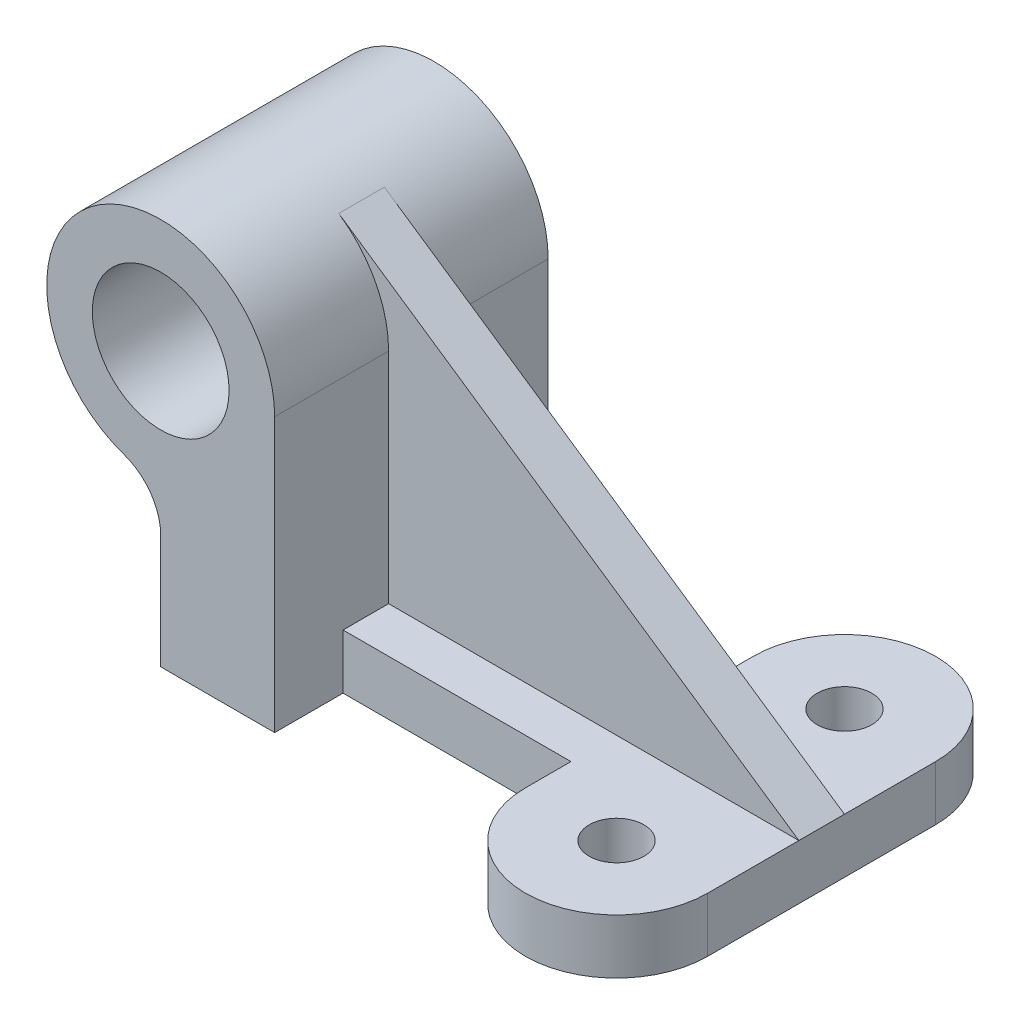
ISO-10303-21;
HEADER;
FILE_DESCRIPTION(('STEP AP214'),'2;1');
FILE_NAME('part.step','',(''),(''),'','','');
FILE_SCHEMA(('AUTOMOTIVE_DESIGN { 1 0 10303 214 1 1 1 1 }'));
ENDSEC;
DATA;
#1=APPLICATION_CONTEXT('core data for automotive mechanical design processes');
#2=APPLICATION_PROTOCOL_DEFINITION('international standard','automotive_design',2000,#1);
#3=PRODUCT_CONTEXT('',#1,'mechanical');
#4=PRODUCT('Part','Part','',(#3));
#5=PRODUCT_RELATED_PRODUCT_CATEGORY('part','',(#4));
#6=PRODUCT_DEFINITION_FORMATION('','',#4);
#7=PRODUCT_DEFINITION_CONTEXT('part definition',#1,'design');
#8=PRODUCT_DEFINITION('design','',#6,#7);
#9=PRODUCT_DEFINITION_SHAPE('','',#8);
#10=(LENGTH_UNIT() NAMED_UNIT(*) SI_UNIT(.MILLI.,.METRE.));
#11=(NAMED_UNIT(*) PLANE_ANGLE_UNIT() SI_UNIT($,.RADIAN.));
#12=(NAMED_UNIT(*) SI_UNIT($,.STERADIAN.) SOLID_ANGLE_UNIT());
#13=UNCERTAINTY_MEASURE_WITH_UNIT(LENGTH_MEASURE(1.E-05),#10,'distance_accuracy_value','');
#14=(GEOMETRIC_REPRESENTATION_CONTEXT(3) GLOBAL_UNCERTAINTY_ASSIGNED_CONTEXT((#13)) GLOBAL_UNIT_ASSIGNED_CONTEXT((#10,
#11,#12)) REPRESENTATION_CONTEXT('',''));
#15=CARTESIAN_POINT('',(0.,0.,0.));
#16=DIRECTION('',(0.,0.,1.));
#17=DIRECTION('',(1.,0.,0.));
#18=AXIS2_PLACEMENT_3D('',#15,#16,#17);
#19=CARTESIAN_POINT('',(0.,6.,25.));
#20=DIRECTION('',(0.,1.,0.));
#21=DIRECTION('',(0.,0.,1.));
#22=AXIS2_PLACEMENT_3D('',#19,#20,#21);
#23=PLANE('',#22);
#24=CARTESIAN_POINT('',(0.,6.,-25.));
#25=DIRECTION('',(0.,1.,0.));
#26=DIRECTION('',(0.,0.,1.));
#27=AXIS2_PLACEMENT_3D('',#24,#25,#26);
#28=CIRCLE('',#27,6.);
#29=CARTESIAN_POINT('',(0.,6.,-19.));
#30=VERTEX_POINT('',#29);
#31=EDGE_CURVE('E241',#30,#30,#28,.T.);
#32=ORIENTED_EDGE('',*,*,#31,.F.);
#33=EDGE_LOOP('',(#32));
#34=FACE_BOUND('',#33,.T.);
#35=DIRECTION('',(0.,0.,1.));
#36=VECTOR('',#35,1.);
#37=CARTESIAN_POINT('',(-70.,6.,-15.));
#38=LINE('',#37,#36);
#39=CARTESIAN_POINT('',(-70.,6.,-15.));
#40=VERTEX_POINT('',#39);
#41=CARTESIAN_POINT('',(-70.,6.,-5.));
#42=VERTEX_POINT('',#41);
#43=EDGE_CURVE('E259',#40,#42,#38,.T.);
#44=ORIENTED_EDGE('',*,*,#43,.T.);
#45=DIRECTION('',(1.,0.,0.));
#46=VECTOR('',#45,1.);
#47=CARTESIAN_POINT('',(0.,6.,-5.));
#48=LINE('',#47,#46);
#49=CARTESIAN_POINT('',(20.,6.,-5.));
#50=VERTEX_POINT('',#49);
#51=EDGE_CURVE('E59',#42,#50,#48,.T.);
#52=ORIENTED_EDGE('',*,*,#51,.T.);
#53=DIRECTION('',(0.,0.,-1.));
#54=VECTOR('',#53,1.);
#55=CARTESIAN_POINT('',(20.,6.,-25.));
#56=LINE('',#55,#54);
#57=CARTESIAN_POINT('',(20.,6.,-25.));
#58=VERTEX_POINT('',#57);
#59=EDGE_CURVE('E270',#50,#58,#56,.T.);
#60=ORIENTED_EDGE('',*,*,#59,.T.);
#61=CARTESIAN_POINT('',(0.,6.,-25.));
#62=DIRECTION('',(0.,1.,0.));
#63=DIRECTION('',(0.,0.,1.));
#64=AXIS2_PLACEMENT_3D('',#61,#62,#63);
#65=CIRCLE('',#64,20.);
#66=CARTESIAN_POINT('',(-20.,6.,-25.));
#67=VERTEX_POINT('',#66);
#68=EDGE_CURVE('E269',#58,#67,#65,.T.);
#69=ORIENTED_EDGE('',*,*,#68,.T.);
#70=DIRECTION('',(0.,0.,1.));
#71=VECTOR('',#70,1.);
#72=CARTESIAN_POINT('',(-20.,6.,-25.));
#73=LINE('',#72,#71);
#74=CARTESIAN_POINT('',(-20.,6.,-15.));
#75=VERTEX_POINT('',#74);
#76=EDGE_CURVE('E253',#67,#75,#73,.T.);
#77=ORIENTED_EDGE('',*,*,#76,.T.);
#78=DIRECTION('',(-1.,0.,0.));
#79=VECTOR('',#78,1.);
#80=CARTESIAN_POINT('',(-70.,6.,-15.));
#81=LINE('',#80,#79);
#82=EDGE_CURVE('E255',#75,#40,#81,.T.);
#83=ORIENTED_EDGE('',*,*,#82,.T.);
#84=EDGE_LOOP('',(#44,#52,#60,#69,#77,#83));
#85=FACE_BOUND('',#84,.T.);
#86=ADVANCED_FACE('F43',(#34,#85),#23,.T.);
#87=CARTESIAN_POINT('',(-70.,-6.,30.));
#88=DIRECTION('',(-1.,0.,0.));
#89=DIRECTION('',(0.,0.,1.));
#90=AXIS2_PLACEMENT_3D('',#87,#88,#89);
#91=PLANE('',#90);
#92=DIRECTION('',(0.,1.,0.));
#93=VECTOR('',#92,1.);
#94=CARTESIAN_POINT('',(-70.,-6.,-5.));
#95=LINE('',#94,#93);
#96=CARTESIAN_POINT('',(-70.,54.,-5.));
#97=VERTEX_POINT('',#96);
#98=EDGE_CURVE('E177',#42,#97,#95,.T.);
#99=ORIENTED_EDGE('',*,*,#98,.F.);
#100=ORIENTED_EDGE('',*,*,#43,.F.);
#101=DIRECTION('',(0.,-1.,0.));
#102=VECTOR('',#101,1.);
#103=CARTESIAN_POINT('',(-70.,6.,-15.));
#104=LINE('',#103,#102);
#105=CARTESIAN_POINT('',(-70.,-6.,-15.));
#106=VERTEX_POINT('',#105);
#107=EDGE_CURVE('E303',#40,#106,#104,.T.);
#108=ORIENTED_EDGE('',*,*,#107,.T.);
#109=DIRECTION('',(0.,0.,-1.));
#110=VECTOR('',#109,1.);
#111=CARTESIAN_POINT('',(-70.,-6.,30.));
#112=LINE('',#111,#110);
#113=CARTESIAN_POINT('',(-70.,-6.,-30.));
#114=VERTEX_POINT('',#113);
#115=EDGE_CURVE('E213',#106,#114,#112,.T.);
#116=ORIENTED_EDGE('',*,*,#115,.T.);
#117=DIRECTION('',(0.,1.,0.));
#118=VECTOR('',#117,1.);
#119=CARTESIAN_POINT('',(-70.,-6.,-30.));
#120=LINE('',#119,#118);
#121=CARTESIAN_POINT('',(-70.,54.,-30.));
#122=VERTEX_POINT('',#121);
#123=EDGE_CURVE('E196',#114,#122,#120,.T.);
#124=ORIENTED_EDGE('',*,*,#123,.T.);
#125=DIRECTION('',(0.,0.,-1.));
#126=VECTOR('',#125,1.);
#127=CARTESIAN_POINT('',(-70.,54.,30.));
#128=LINE('',#127,#126);
#129=EDGE_CURVE('E234',#97,#122,#128,.T.);
#130=ORIENTED_EDGE('',*,*,#129,.F.);
#131=EDGE_LOOP('',(#99,#100,#108,#116,#124,#130));
#132=FACE_BOUND('',#131,.T.);
#133=ADVANCED_FACE('F323',(#132),#91,.F.);
#134=DIRECTION('',(1.,0.,0.));
#135=VECTOR('',#134,1.);
#136=CARTESIAN_POINT('',(0.,6.,5.));
#137=LINE('',#136,#135);
#138=CARTESIAN_POINT('',(-70.,6.,5.));
#139=VERTEX_POINT('',#138);
#140=CARTESIAN_POINT('',(20.,6.,5.));
#141=VERTEX_POINT('',#140);
#142=EDGE_CURVE('E186',#139,#141,#137,.T.);
#143=ORIENTED_EDGE('',*,*,#142,.F.);
#144=CARTESIAN_POINT('',(-70.,6.,15.));
#145=VERTEX_POINT('',#144);
#146=EDGE_CURVE('E256',#139,#145,#38,.T.);
#147=ORIENTED_EDGE('',*,*,#146,.T.);
#148=DIRECTION('',(1.,0.,0.));
#149=VECTOR('',#148,1.);
#150=CARTESIAN_POINT('',(-70.,6.,15.));
#151=LINE('',#150,#149);
#152=CARTESIAN_POINT('',(-20.,6.,15.));
#153=VERTEX_POINT('',#152);
#154=EDGE_CURVE('E261',#145,#153,#151,.T.);
#155=ORIENTED_EDGE('',*,*,#154,.T.);
#156=DIRECTION('',(0.,0.,1.));
#157=VECTOR('',#156,1.);
#158=CARTESIAN_POINT('',(-20.,6.,15.));
#159=LINE('',#158,#157);
#160=CARTESIAN_POINT('',(-20.,6.,25.));
#161=VERTEX_POINT('',#160);
#162=EDGE_CURVE('E263',#153,#161,#159,.T.);
#163=ORIENTED_EDGE('',*,*,#162,.T.);
#164=CARTESIAN_POINT('',(0.,6.,25.));
#165=DIRECTION('',(0.,1.,0.));
#166=DIRECTION('',(0.,0.,1.));
#167=AXIS2_PLACEMENT_3D('',#164,#165,#166);
#168=CIRCLE('',#167,20.);
#169=CARTESIAN_POINT('',(20.,6.,25.));
#170=VERTEX_POINT('',#169);
#171=EDGE_CURVE('E264',#161,#170,#168,.T.);
#172=ORIENTED_EDGE('',*,*,#171,.T.);
#173=EDGE_CURVE('E268',#170,#141,#56,.T.);
#174=ORIENTED_EDGE('',*,*,#173,.T.);
#175=EDGE_LOOP('',(#143,#147,#155,#163,#172,#174));
#176=FACE_BOUND('',#175,.T.);
#177=CARTESIAN_POINT('',(0.,6.,25.));
#178=DIRECTION('',(0.,1.,0.));
#179=DIRECTION('',(0.,0.,1.));
#180=AXIS2_PLACEMENT_3D('',#177,#178,#179);
#181=CIRCLE('',#180,6.);
#182=CARTESIAN_POINT('',(0.,6.,31.));
#183=VERTEX_POINT('',#182);
#184=EDGE_CURVE('E239',#183,#183,#181,.T.);
#185=ORIENTED_EDGE('',*,*,#184,.F.);
#186=EDGE_LOOP('',(#185));
#187=FACE_BOUND('',#186,.T.);
#188=ADVANCED_FACE('F385',(#176,#187),#23,.T.);
#189=CARTESIAN_POINT('',(0.,-6.,25.));
#190=DIRECTION('',(0.,1.,0.));
#191=DIRECTION('',(0.,0.,1.));
#192=AXIS2_PLACEMENT_3D('',#189,#190,#191);
#193=PLANE('',#192);
#194=DIRECTION('',(0.,0.,-1.));
#195=VECTOR('',#194,1.);
#196=CARTESIAN_POINT('',(-95.,-6.,30.));
#197=LINE('',#196,#195);
#198=CARTESIAN_POINT('',(-95.,-6.,30.));
#199=VERTEX_POINT('',#198);
#200=CARTESIAN_POINT('',(-95.,-6.,-30.));
#201=VERTEX_POINT('',#200);
#202=EDGE_CURVE('E230',#199,#201,#197,.T.);
#203=ORIENTED_EDGE('',*,*,#202,.T.);
#204=DIRECTION('',(1.,0.,0.));
#205=VECTOR('',#204,1.);
#206=CARTESIAN_POINT('',(-70.,-6.,-30.));
#207=LINE('',#206,#205);
#208=EDGE_CURVE('E202',#201,#114,#207,.T.);
#209=ORIENTED_EDGE('',*,*,#208,.T.);
#210=ORIENTED_EDGE('',*,*,#115,.F.);
#211=DIRECTION('',(-1.,0.,0.));
#212=VECTOR('',#211,1.);
#213=CARTESIAN_POINT('',(-70.,-6.,-15.));
#214=LINE('',#213,#212);
#215=CARTESIAN_POINT('',(-20.,-6.,-15.));
#216=VERTEX_POINT('',#215);
#217=EDGE_CURVE('E274',#216,#106,#214,.T.);
#218=ORIENTED_EDGE('',*,*,#217,.F.);
#219=DIRECTION('',(0.,0.,1.));
#220=VECTOR('',#219,1.);
#221=CARTESIAN_POINT('',(-20.,-6.,-25.));
#222=LINE('',#221,#220);
#223=CARTESIAN_POINT('',(-20.,-6.,-25.));
#224=VERTEX_POINT('',#223);
#225=EDGE_CURVE('E247',#224,#216,#222,.T.);
#226=ORIENTED_EDGE('',*,*,#225,.F.);
#227=CARTESIAN_POINT('',(0.,-6.,-25.));
#228=DIRECTION('',(0.,1.,0.));
#229=DIRECTION('',(0.,0.,1.));
#230=AXIS2_PLACEMENT_3D('',#227,#228,#229);
#231=CIRCLE('',#230,20.);
#232=CARTESIAN_POINT('',(20.,-6.,-25.));
#233=VERTEX_POINT('',#232);
#234=EDGE_CURVE('E254',#233,#224,#231,.T.);
#235=ORIENTED_EDGE('',*,*,#234,.F.);
#236=DIRECTION('',(0.,0.,-1.));
#237=VECTOR('',#236,1.);
#238=CARTESIAN_POINT('',(20.,-6.,-25.));
#239=LINE('',#238,#237);
#240=CARTESIAN_POINT('',(20.,-6.,25.));
#241=VERTEX_POINT('',#240);
#242=EDGE_CURVE('E285',#241,#233,#239,.T.);
#243=ORIENTED_EDGE('',*,*,#242,.F.);
#244=CARTESIAN_POINT('',(0.,-6.,25.));
#245=DIRECTION('',(0.,1.,0.));
#246=DIRECTION('',(0.,0.,1.));
#247=AXIS2_PLACEMENT_3D('',#244,#245,#246);
#248=CIRCLE('',#247,20.);
#249=CARTESIAN_POINT('',(-20.,-6.,25.));
#250=VERTEX_POINT('',#249);
#251=EDGE_CURVE('E284',#250,#241,#248,.T.);
#252=ORIENTED_EDGE('',*,*,#251,.F.);
#253=DIRECTION('',(0.,0.,1.));
#254=VECTOR('',#253,1.);
#255=CARTESIAN_POINT('',(-20.,-6.,15.));
#256=LINE('',#255,#254);
#257=CARTESIAN_POINT('',(-20.,-6.,15.));
#258=VERTEX_POINT('',#257);
#259=EDGE_CURVE('E278',#258,#250,#256,.T.);
#260=ORIENTED_EDGE('',*,*,#259,.F.);
#261=DIRECTION('',(1.,0.,0.));
#262=VECTOR('',#261,1.);
#263=CARTESIAN_POINT('',(-70.,-6.,15.));
#264=LINE('',#263,#262);
#265=CARTESIAN_POINT('',(-70.,-6.,15.));
#266=VERTEX_POINT('',#265);
#267=EDGE_CURVE('E279',#266,#258,#264,.T.);
#268=ORIENTED_EDGE('',*,*,#267,.F.);
#269=CARTESIAN_POINT('',(-70.,-6.,30.));
#270=VERTEX_POINT('',#269);
#271=EDGE_CURVE('E229',#270,#266,#112,.T.);
#272=ORIENTED_EDGE('',*,*,#271,.F.);
#273=DIRECTION('',(1.,0.,0.));
#274=VECTOR('',#273,1.);
#275=CARTESIAN_POINT('',(-70.,-6.,30.));
#276=LINE('',#275,#274);
#277=EDGE_CURVE('E211',#199,#270,#276,.T.);
#278=ORIENTED_EDGE('',*,*,#277,.F.);
#279=EDGE_LOOP('',(#203,#209,#210,#218,#226,#235,#243,#252,#260,#268,#272,#278));
#280=FACE_BOUND('',#279,.T.);
#281=CARTESIAN_POINT('',(0.,-6.,25.));
#282=DIRECTION('',(0.,1.,0.));
#283=DIRECTION('',(0.,0.,1.));
#284=AXIS2_PLACEMENT_3D('',#281,#282,#283);
#285=CIRCLE('',#284,6.);
#286=CARTESIAN_POINT('',(0.,-6.,31.));
#287=VERTEX_POINT('',#286);
#288=EDGE_CURVE('E236',#287,#287,#285,.T.);
#289=ORIENTED_EDGE('',*,*,#288,.T.);
#290=EDGE_LOOP('',(#289));
#291=FACE_BOUND('',#290,.T.);
#292=CARTESIAN_POINT('',(0.,-6.,-25.));
#293=DIRECTION('',(0.,1.,0.));
#294=DIRECTION('',(0.,0.,1.));
#295=AXIS2_PLACEMENT_3D('',#292,#293,#294);
#296=CIRCLE('',#295,6.);
#297=CARTESIAN_POINT('',(0.,-6.,-19.));
#298=VERTEX_POINT('',#297);
#299=EDGE_CURVE('E244',#298,#298,#296,.T.);
#300=ORIENTED_EDGE('',*,*,#299,.T.);
#301=EDGE_LOOP('',(#300));
#302=FACE_BOUND('',#301,.T.);
#303=ADVANCED_FACE('F316',(#280,#291,#302),#193,.F.);
#304=CARTESIAN_POINT('',(-20.,6.,-25.));
#305=DIRECTION('',(1.,0.,0.));
#306=DIRECTION('',(0.,0.,-1.));
#307=AXIS2_PLACEMENT_3D('',#304,#305,#306);
#308=PLANE('',#307);
#309=ORIENTED_EDGE('',*,*,#225,.T.);
#310=DIRECTION('',(0.,-1.,0.));
#311=VECTOR('',#310,1.);
#312=CARTESIAN_POINT('',(-20.,6.,-15.));
#313=LINE('',#312,#311);
#314=EDGE_CURVE('E51',#75,#216,#313,.T.);
#315=ORIENTED_EDGE('',*,*,#314,.F.);
#316=ORIENTED_EDGE('',*,*,#76,.F.);
#317=DIRECTION('',(0.,-1.,0.));
#318=VECTOR('',#317,1.);
#319=CARTESIAN_POINT('',(-20.,6.,-25.));
#320=LINE('',#319,#318);
#321=EDGE_CURVE('E275',#67,#224,#320,.T.);
#322=ORIENTED_EDGE('',*,*,#321,.T.);
#323=EDGE_LOOP('',(#309,#315,#316,#322));
#324=FACE_BOUND('',#323,.T.);
#325=ADVANCED_FACE('F44',(#324),#308,.F.);
#326=CARTESIAN_POINT('',(-70.,6.,-15.));
#327=DIRECTION('',(0.,0.,1.));
#328=DIRECTION('',(1.,0.,0.));
#329=AXIS2_PLACEMENT_3D('',#326,#327,#328);
#330=PLANE('',#329);
#331=ORIENTED_EDGE('',*,*,#217,.T.);
#332=ORIENTED_EDGE('',*,*,#107,.F.);
#333=ORIENTED_EDGE('',*,*,#82,.F.);
#334=ORIENTED_EDGE('',*,*,#314,.T.);
#335=EDGE_LOOP('',(#331,#332,#333,#334));
#336=FACE_BOUND('',#335,.T.);
#337=ADVANCED_FACE('F306',(#336),#330,.F.);
#338=CARTESIAN_POINT('',(-70.,6.,15.));
#339=DIRECTION('',(0.,0.,-1.));
#340=DIRECTION('',(-1.,0.,0.));
#341=AXIS2_PLACEMENT_3D('',#338,#339,#340);
#342=PLANE('',#341);
#343=ORIENTED_EDGE('',*,*,#267,.T.);
#344=DIRECTION('',(0.,-1.,0.));
#345=VECTOR('',#344,1.);
#346=CARTESIAN_POINT('',(-20.,6.,15.));
#347=LINE('',#346,#345);
#348=EDGE_CURVE('E297',#153,#258,#347,.T.);
#349=ORIENTED_EDGE('',*,*,#348,.F.);
#350=ORIENTED_EDGE('',*,*,#154,.F.);
#351=DIRECTION('',(0.,-1.,0.));
#352=VECTOR('',#351,1.);
#353=CARTESIAN_POINT('',(-70.,6.,15.));
#354=LINE('',#353,#352);
#355=EDGE_CURVE('E301',#145,#266,#354,.T.);
#356=ORIENTED_EDGE('',*,*,#355,.T.);
#357=EDGE_LOOP('',(#343,#349,#350,#356));
#358=FACE_BOUND('',#357,.T.);
#359=ADVANCED_FACE('F342',(#358),#342,.F.);
#360=CARTESIAN_POINT('',(-20.,6.,15.));
#361=DIRECTION('',(1.,0.,0.));
#362=DIRECTION('',(0.,0.,-1.));
#363=AXIS2_PLACEMENT_3D('',#360,#361,#362);
#364=PLANE('',#363);
#365=ORIENTED_EDGE('',*,*,#259,.T.);
#366=DIRECTION('',(0.,-1.,0.));
#367=VECTOR('',#366,1.);
#368=CARTESIAN_POINT('',(-20.,6.,25.));
#369=LINE('',#368,#367);
#370=EDGE_CURVE('E293',#161,#250,#369,.T.);
#371=ORIENTED_EDGE('',*,*,#370,.F.);
#372=ORIENTED_EDGE('',*,*,#162,.F.);
#373=ORIENTED_EDGE('',*,*,#348,.T.);
#374=EDGE_LOOP('',(#365,#371,#372,#373));
#375=FACE_BOUND('',#374,.T.);
#376=ADVANCED_FACE('F340',(#375),#364,.F.);
#377=CARTESIAN_POINT('',(0.,6.,25.));
#378=DIRECTION('',(0.,-1.,0.));
#379=DIRECTION('',(0.,0.,-1.));
#380=AXIS2_PLACEMENT_3D('',#377,#378,#379);
#381=CYLINDRICAL_SURFACE('',#380,20.);
#382=ORIENTED_EDGE('',*,*,#251,.T.);
#383=DIRECTION('',(0.,-1.,0.));
#384=VECTOR('',#383,1.);
#385=CARTESIAN_POINT('',(20.,6.,25.));
#386=LINE('',#385,#384);
#387=EDGE_CURVE('E295',#170,#241,#386,.T.);
#388=ORIENTED_EDGE('',*,*,#387,.F.);
#389=ORIENTED_EDGE('',*,*,#171,.F.);
#390=ORIENTED_EDGE('',*,*,#370,.T.);
#391=EDGE_LOOP('',(#382,#388,#389,#390));
#392=FACE_BOUND('',#391,.T.);
#393=ADVANCED_FACE('F331',(#392),#381,.T.);
#394=CARTESIAN_POINT('',(20.,6.,-25.));
#395=DIRECTION('',(-1.,0.,0.));
#396=DIRECTION('',(0.,0.,1.));
#397=AXIS2_PLACEMENT_3D('',#394,#395,#396);
#398=PLANE('',#397);
#399=ORIENTED_EDGE('',*,*,#242,.T.);
#400=DIRECTION('',(0.,-1.,0.));
#401=VECTOR('',#400,1.);
#402=CARTESIAN_POINT('',(20.,6.,-25.));
#403=LINE('',#402,#401);
#404=EDGE_CURVE('E288',#58,#233,#403,.T.);
#405=ORIENTED_EDGE('',*,*,#404,.F.);
#406=ORIENTED_EDGE('',*,*,#59,.F.);
#407=DIRECTION('',(0.,0.,-1.));
#408=VECTOR('',#407,1.);
#409=CARTESIAN_POINT('',(20.,6.,-25.));
#410=LINE('',#409,#408);
#411=EDGE_CURVE('E61',#141,#50,#410,.T.);
#412=ORIENTED_EDGE('',*,*,#411,.F.);
#413=ORIENTED_EDGE('',*,*,#173,.F.);
#414=ORIENTED_EDGE('',*,*,#387,.T.);
#415=EDGE_LOOP('',(#399,#405,#406,#412,#413,#414));
#416=FACE_BOUND('',#415,.T.);
#417=ADVANCED_FACE('F327',(#416),#398,.F.);
#418=CARTESIAN_POINT('',(0.,6.,-25.));
#419=DIRECTION('',(0.,-1.,0.));
#420=DIRECTION('',(0.,0.,-1.));
#421=AXIS2_PLACEMENT_3D('',#418,#419,#420);
#422=CYLINDRICAL_SURFACE('',#421,20.);
#423=ORIENTED_EDGE('',*,*,#234,.T.);
#424=ORIENTED_EDGE('',*,*,#321,.F.);
#425=ORIENTED_EDGE('',*,*,#68,.F.);
#426=ORIENTED_EDGE('',*,*,#404,.T.);
#427=EDGE_LOOP('',(#423,#424,#425,#426));
#428=FACE_BOUND('',#427,.T.);
#429=ADVANCED_FACE('F330',(#428),#422,.T.);
#430=CARTESIAN_POINT('',(0.,6.,-25.));
#431=DIRECTION('',(0.,-1.,0.));
#432=DIRECTION('',(0.,0.,-1.));
#433=AXIS2_PLACEMENT_3D('',#430,#431,#432);
#434=CYLINDRICAL_SURFACE('',#433,6.);
#435=ORIENTED_EDGE('',*,*,#31,.T.);
#436=EDGE_LOOP('',(#435));
#437=FACE_BOUND('',#436,.T.);
#438=ORIENTED_EDGE('',*,*,#299,.F.);
#439=EDGE_LOOP('',(#438));
#440=FACE_BOUND('',#439,.T.);
#441=ADVANCED_FACE('F404',(#437,#440),#434,.F.);
#442=CARTESIAN_POINT('',(0.,6.,25.));
#443=DIRECTION('',(0.,-1.,0.));
#444=DIRECTION('',(0.,0.,-1.));
#445=AXIS2_PLACEMENT_3D('',#442,#443,#444);
#446=CYLINDRICAL_SURFACE('',#445,6.);
#447=ORIENTED_EDGE('',*,*,#184,.T.);
#448=EDGE_LOOP('',(#447));
#449=FACE_BOUND('',#448,.T.);
#450=ORIENTED_EDGE('',*,*,#288,.F.);
#451=EDGE_LOOP('',(#450));
#452=FACE_BOUND('',#451,.T.);
#453=ADVANCED_FACE('F402',(#449,#452),#446,.F.);
#454=ORIENTED_EDGE('',*,*,#146,.F.);
#455=DIRECTION('',(0.,1.,0.));
#456=VECTOR('',#455,1.);
#457=CARTESIAN_POINT('',(-70.,-6.,5.));
#458=LINE('',#457,#456);
#459=CARTESIAN_POINT('',(-70.,54.,5.));
#460=VERTEX_POINT('',#459);
#461=EDGE_CURVE('E187',#139,#460,#458,.T.);
#462=ORIENTED_EDGE('',*,*,#461,.T.);
#463=CARTESIAN_POINT('',(-70.,54.,30.));
#464=VERTEX_POINT('',#463);
#465=EDGE_CURVE('E237',#464,#460,#128,.T.);
#466=ORIENTED_EDGE('',*,*,#465,.F.);
#467=DIRECTION('',(0.,1.,0.));
#468=VECTOR('',#467,1.);
#469=CARTESIAN_POINT('',(-70.,-6.,30.));
#470=LINE('',#469,#468);
#471=EDGE_CURVE('E203',#270,#464,#470,.T.);
#472=ORIENTED_EDGE('',*,*,#471,.F.);
#473=ORIENTED_EDGE('',*,*,#271,.T.);
#474=ORIENTED_EDGE('',*,*,#355,.F.);
#475=EDGE_LOOP('',(#454,#462,#466,#472,#473,#474));
#476=FACE_BOUND('',#475,.T.);
#477=ADVANCED_FACE('F353',(#476),#91,.F.);
#478=CARTESIAN_POINT('',(-95.,54.,30.));
#479=DIRECTION('',(0.,0.,1.));
#480=DIRECTION('',(1.,0.,0.));
#481=AXIS2_PLACEMENT_3D('',#478,#479,#480);
#482=PLANE('',#481);
#483=ORIENTED_EDGE('',*,*,#471,.T.);
#484=CARTESIAN_POINT('',(-95.,54.,30.));
#485=DIRECTION('',(0.,0.,1.));
#486=DIRECTION('',(1.,0.,0.));
#487=AXIS2_PLACEMENT_3D('',#484,#485,#486);
#488=CIRCLE('',#487,25.);
#489=CARTESIAN_POINT('',(-103.108108108108,30.3513513513513,30.));
#490=VERTEX_POINT('',#489);
#491=EDGE_CURVE('E204',#464,#490,#488,.T.);
#492=ORIENTED_EDGE('',*,*,#491,.T.);
#493=CARTESIAN_POINT('',(-107.,19.,30.));
#494=DIRECTION('',(0.,0.,-1.));
#495=DIRECTION('',(1.,0.,0.));
#496=AXIS2_PLACEMENT_3D('',#493,#494,#495);
#497=CIRCLE('',#496,12.);
#498=CARTESIAN_POINT('',(-95.,19.,30.));
#499=VERTEX_POINT('',#498);
#500=EDGE_CURVE('E210',#490,#499,#497,.T.);
#501=ORIENTED_EDGE('',*,*,#500,.T.);
#502=DIRECTION('',(0.,-1.,0.));
#503=VECTOR('',#502,1.);
#504=CARTESIAN_POINT('',(-95.,-6.,30.));
#505=LINE('',#504,#503);
#506=EDGE_CURVE('E207',#499,#199,#505,.T.);
#507=ORIENTED_EDGE('',*,*,#506,.T.);
#508=ORIENTED_EDGE('',*,*,#277,.T.);
#509=EDGE_LOOP('',(#483,#492,#501,#507,#508));
#510=FACE_BOUND('',#509,.T.);
#511=CARTESIAN_POINT('',(-95.,54.,30.));
#512=DIRECTION('',(0.,0.,1.));
#513=DIRECTION('',(1.,0.,0.));
#514=AXIS2_PLACEMENT_3D('',#511,#512,#513);
#515=CIRCLE('',#514,15.);
#516=CARTESIAN_POINT('',(-80.,54.,30.));
#517=VERTEX_POINT('',#516);
#518=EDGE_CURVE('E194',#517,#517,#515,.T.);
#519=ORIENTED_EDGE('',*,*,#518,.F.);
#520=EDGE_LOOP('',(#519));
#521=FACE_BOUND('',#520,.T.);
#522=ADVANCED_FACE('F352',(#510,#521),#482,.T.);
#523=CARTESIAN_POINT('',(-95.,54.,-30.));
#524=DIRECTION('',(0.,0.,1.));
#525=DIRECTION('',(1.,0.,0.));
#526=AXIS2_PLACEMENT_3D('',#523,#524,#525);
#527=PLANE('',#526);
#528=ORIENTED_EDGE('',*,*,#123,.F.);
#529=ORIENTED_EDGE('',*,*,#208,.F.);
#530=DIRECTION('',(0.,-1.,0.));
#531=VECTOR('',#530,1.);
#532=CARTESIAN_POINT('',(-95.,-6.,-30.));
#533=LINE('',#532,#531);
#534=CARTESIAN_POINT('',(-95.,19.,-30.));
#535=VERTEX_POINT('',#534);
#536=EDGE_CURVE('E225',#535,#201,#533,.T.);
#537=ORIENTED_EDGE('',*,*,#536,.F.);
#538=CARTESIAN_POINT('',(-107.,19.,-30.));
#539=DIRECTION('',(0.,0.,-1.));
#540=DIRECTION('',(1.,0.,0.));
#541=AXIS2_PLACEMENT_3D('',#538,#539,#540);
#542=CIRCLE('',#541,12.);
#543=CARTESIAN_POINT('',(-103.108108108108,30.3513513513513,-30.));
#544=VERTEX_POINT('',#543);
#545=EDGE_CURVE('E218',#544,#535,#542,.T.);
#546=ORIENTED_EDGE('',*,*,#545,.F.);
#547=CARTESIAN_POINT('',(-95.,54.,-30.));
#548=DIRECTION('',(0.,0.,1.));
#549=DIRECTION('',(1.,0.,0.));
#550=AXIS2_PLACEMENT_3D('',#547,#548,#549);
#551=CIRCLE('',#550,25.);
#552=EDGE_CURVE('E216',#122,#544,#551,.T.);
#553=ORIENTED_EDGE('',*,*,#552,.F.);
#554=EDGE_LOOP('',(#528,#529,#537,#546,#553));
#555=FACE_BOUND('',#554,.T.);
#556=CARTESIAN_POINT('',(-95.,54.,-30.));
#557=DIRECTION('',(0.,0.,1.));
#558=DIRECTION('',(1.,0.,0.));
#559=AXIS2_PLACEMENT_3D('',#556,#557,#558);
#560=CIRCLE('',#559,15.);
#561=CARTESIAN_POINT('',(-80.,54.,-30.));
#562=VERTEX_POINT('',#561);
#563=EDGE_CURVE('E193',#562,#562,#560,.T.);
#564=ORIENTED_EDGE('',*,*,#563,.T.);
#565=EDGE_LOOP('',(#564));
#566=FACE_BOUND('',#565,.T.);
#567=ADVANCED_FACE('F364',(#555,#566),#527,.F.);
#568=CARTESIAN_POINT('',(-95.,54.,30.));
#569=DIRECTION('',(0.,0.,-1.));
#570=DIRECTION('',(-1.,0.,0.));
#571=AXIS2_PLACEMENT_3D('',#568,#569,#570);
#572=CYLINDRICAL_SURFACE('',#571,25.);
#573=CARTESIAN_POINT('',(-95.,54.,5.));
#574=DIRECTION('',(0.,0.,1.));
#575=DIRECTION('',(1.,0.,0.));
#576=AXIS2_PLACEMENT_3D('',#573,#574,#575);
#577=CIRCLE('',#576,25.);
#578=CARTESIAN_POINT('',(-80.9377083111916,74.6700738377701,5.));
#579=VERTEX_POINT('',#578);
#580=EDGE_CURVE('E169',#460,#579,#577,.T.);
#581=ORIENTED_EDGE('',*,*,#580,.T.);
#582=DIRECTION('',(0.,0.,-1.));
#583=VECTOR('',#582,1.);
#584=CARTESIAN_POINT('',(-80.9377083111916,74.6700738377702,30.));
#585=LINE('',#584,#583);
#586=CARTESIAN_POINT('',(-80.9377083111916,74.6700738377701,-5.));
#587=VERTEX_POINT('',#586);
#588=EDGE_CURVE('E11',#579,#587,#585,.T.);
#589=ORIENTED_EDGE('',*,*,#588,.T.);
#590=CARTESIAN_POINT('',(-95.,54.,-5.));
#591=DIRECTION('',(0.,0.,1.));
#592=DIRECTION('',(1.,0.,0.));
#593=AXIS2_PLACEMENT_3D('',#590,#591,#592);
#594=CIRCLE('',#593,25.);
#595=EDGE_CURVE('E163',#97,#587,#594,.T.);
#596=ORIENTED_EDGE('',*,*,#595,.F.);
#597=ORIENTED_EDGE('',*,*,#129,.T.);
#598=ORIENTED_EDGE('',*,*,#552,.T.);
#599=DIRECTION('',(0.,0.,-1.));
#600=VECTOR('',#599,1.);
#601=CARTESIAN_POINT('',(-103.108108108108,30.3513513513513,30.));
#602=LINE('',#601,#600);
#603=EDGE_CURVE('E232',#490,#544,#602,.T.);
#604=ORIENTED_EDGE('',*,*,#603,.F.);
#605=ORIENTED_EDGE('',*,*,#491,.F.);
#606=ORIENTED_EDGE('',*,*,#465,.T.);
#607=EDGE_LOOP('',(#581,#589,#596,#597,#598,#604,#605,#606));
#608=FACE_BOUND('',#607,.T.);
#609=ADVANCED_FACE('F162',(#608),#572,.T.);
#610=CARTESIAN_POINT('',(-107.,19.,30.));
#611=DIRECTION('',(0.,0.,-1.));
#612=DIRECTION('',(-1.,0.,0.));
#613=AXIS2_PLACEMENT_3D('',#610,#611,#612);
#614=CYLINDRICAL_SURFACE('',#613,12.);
#615=ORIENTED_EDGE('',*,*,#603,.T.);
#616=ORIENTED_EDGE('',*,*,#545,.T.);
#617=DIRECTION('',(0.,0.,-1.));
#618=VECTOR('',#617,1.);
#619=CARTESIAN_POINT('',(-95.,19.,30.));
#620=LINE('',#619,#618);
#621=EDGE_CURVE('E231',#499,#535,#620,.T.);
#622=ORIENTED_EDGE('',*,*,#621,.F.);
#623=ORIENTED_EDGE('',*,*,#500,.F.);
#624=EDGE_LOOP('',(#615,#616,#622,#623));
#625=FACE_BOUND('',#624,.T.);
#626=ADVANCED_FACE('F369',(#625),#614,.F.);
#627=CARTESIAN_POINT('',(-95.,-6.,30.));
#628=DIRECTION('',(1.,0.,0.));
#629=DIRECTION('',(0.,0.,-1.));
#630=AXIS2_PLACEMENT_3D('',#627,#628,#629);
#631=PLANE('',#630);
#632=ORIENTED_EDGE('',*,*,#621,.T.);
#633=ORIENTED_EDGE('',*,*,#536,.T.);
#634=ORIENTED_EDGE('',*,*,#202,.F.);
#635=ORIENTED_EDGE('',*,*,#506,.F.);
#636=EDGE_LOOP('',(#632,#633,#634,#635));
#637=FACE_BOUND('',#636,.T.);
#638=ADVANCED_FACE('F363',(#637),#631,.F.);
#639=CARTESIAN_POINT('',(-95.,54.,30.));
#640=DIRECTION('',(0.,0.,-1.));
#641=DIRECTION('',(-1.,0.,0.));
#642=AXIS2_PLACEMENT_3D('',#639,#640,#641);
#643=CYLINDRICAL_SURFACE('',#642,15.);
#644=ORIENTED_EDGE('',*,*,#518,.T.);
#645=EDGE_LOOP('',(#644));
#646=FACE_BOUND('',#645,.T.);
#647=ORIENTED_EDGE('',*,*,#563,.F.);
#648=EDGE_LOOP('',(#647));
#649=FACE_BOUND('',#648,.T.);
#650=ADVANCED_FACE('F376',(#646,#649),#643,.F.);
#651=CARTESIAN_POINT('',(20.,6.,0.));
#652=DIRECTION('',(0.562491667552336,0.826802953510806,0.));
#653=DIRECTION('',(-0.826802953510806,0.562491667552336,0.));
#654=AXIS2_PLACEMENT_3D('',#651,#652,#653);
#655=PLANE('',#654);
#656=DIRECTION('',(-0.826802953510806,0.562491667552336,0.));
#657=VECTOR('',#656,1.);
#658=CARTESIAN_POINT('',(20.,6.,5.));
#659=LINE('',#658,#657);
#660=EDGE_CURVE('E178',#141,#579,#659,.T.);
#661=ORIENTED_EDGE('',*,*,#660,.F.);
#662=ORIENTED_EDGE('',*,*,#411,.T.);
#663=DIRECTION('',(-0.826802953510806,0.562491667552336,0.));
#664=VECTOR('',#663,1.);
#665=CARTESIAN_POINT('',(20.,6.,-5.));
#666=LINE('',#665,#664);
#667=EDGE_CURVE('E180',#50,#587,#666,.T.);
#668=ORIENTED_EDGE('',*,*,#667,.T.);
#669=ORIENTED_EDGE('',*,*,#588,.F.);
#670=EDGE_LOOP('',(#661,#662,#668,#669));
#671=FACE_BOUND('',#670,.T.);
#672=ADVANCED_FACE('F182',(#671),#655,.T.);
#673=CARTESIAN_POINT('',(-50.,36.5,5.));
#674=DIRECTION('',(0.,0.,1.));
#675=DIRECTION('',(1.,0.,0.));
#676=AXIS2_PLACEMENT_3D('',#673,#674,#675);
#677=PLANE('',#676);
#678=ORIENTED_EDGE('',*,*,#461,.F.);
#679=ORIENTED_EDGE('',*,*,#142,.T.);
#680=ORIENTED_EDGE('',*,*,#660,.T.);
#681=ORIENTED_EDGE('',*,*,#580,.F.);
#682=EDGE_LOOP('',(#678,#679,#680,#681));
#683=FACE_BOUND('',#682,.T.);
#684=ADVANCED_FACE('F431',(#683),#677,.T.);
#685=CARTESIAN_POINT('',(-50.,36.5,-5.));
#686=DIRECTION('',(0.,0.,1.));
#687=DIRECTION('',(1.,0.,0.));
#688=AXIS2_PLACEMENT_3D('',#685,#686,#687);
#689=PLANE('',#688);
#690=ORIENTED_EDGE('',*,*,#51,.F.);
#691=ORIENTED_EDGE('',*,*,#98,.T.);
#692=ORIENTED_EDGE('',*,*,#595,.T.);
#693=ORIENTED_EDGE('',*,*,#667,.F.);
#694=EDGE_LOOP('',(#690,#691,#692,#693));
#695=FACE_BOUND('',#694,.T.);
#696=ADVANCED_FACE('F176',(#695),#689,.F.);
#697=CLOSED_SHELL('',(#86,#133,#188,#303,#325,#337,#359,#376,#393,#417,#429,#441,#453,#477,#522,
#567,#609,#626,#638,#650,#672,#684,#696));
#698=MANIFOLD_SOLID_BREP('B2',#697);
#699=ADVANCED_BREP_SHAPE_REPRESENTATION('',(#18,#698),#14);
#700=SHAPE_DEFINITION_REPRESENTATION(#9,#699);
ENDSEC;
END-ISO-10303-21;
